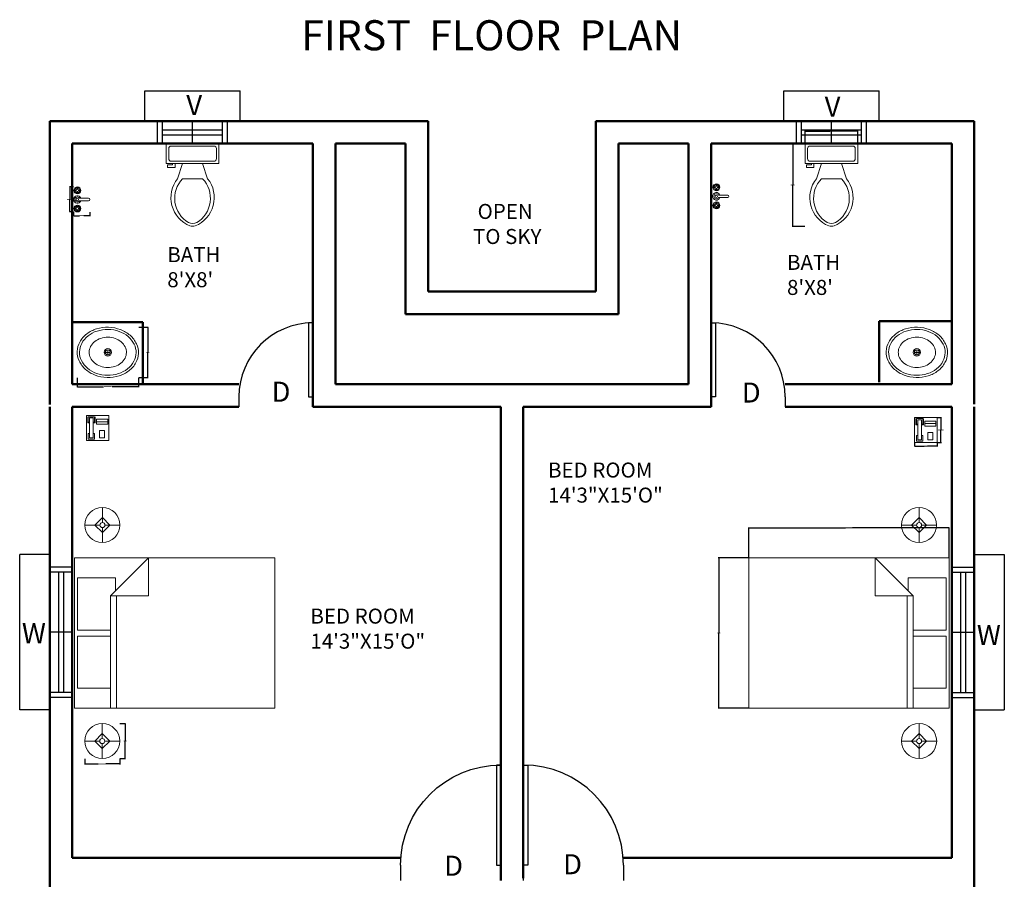
# Model space of a CAD drawing. Units: inches. Extents: x -8 to 1354, y -679 to 94.
# Tile 6 of 6: x 961 to 1354, y -249 to 94. Entities that reach past the tile are written whole.
import ezdxf

# ---------------------------------------------------------------- set-up
doc = ezdxf.new("R2010")
doc.units = ezdxf.units.IN
doc.header["$MEASUREMENT"] = 0
for name, color, linetype, lineweight in [('A-ANNO-DIMS', 2, 'Continuous', 18), ('A-ANNO-TEXT', 7, 'Continuous', 25), ('A-AREA-IDEN', 7, 'Continuous', 25), ('A-DOOR', 3, 'Continuous', 25), ('A-FLOR-FIXT', 8, 'Continuous', 18), ('A-FURN', 8, 'Continuous', 18), ('A-GLAZ', 4, 'Continuous', 25), ('A-WALL', 1, 'Continuous', 50)]:
    doc.layers.add(name, color=color, linetype=linetype, lineweight=lineweight)
doc.styles.get("Standard").update_dxf_attribs({"font": 'arial.ttf'})
doc.dimstyles.get("Standard").update_dxf_attribs({"dimtxt": 0.18, "dimasz": 0.18, "dimexe": 0.18, "dimexo": 0.0625, "dimgap": 0.09, "dimtad": 0, "dimtih": 1, "dimtoh": 1, "dimdec": 1, "dimzin": 0, "dimdsep": 46, "dimlunit": 4, "dimtxsty": 'Standard', "dimcen": 0.09, "dimclrd": 2, "dimclre": 3, "dimclrt": 6, "dimadec": 0, "dimazin": 0, "dimtfac": 1, "dimtdec": 1, "dimtofl": 0, "dimtmove": 0, "dimatfit": 3, "dimfxl": 1, "dimtfill": 2, "dimtfillclr": 4, "dimtolj": 1, "dimtzin": 0, "dimarcsym": 0})

# ---------------------------------------------------------------- blocks, each defined once
blk = doc.blocks.new('*U30')
for p, q in [((0, 0), (0, -6)), ((40, 0), (40, -6))]:
    blk.add_line(p, q)
blk.add_lwpolyline([(0, 0), (0, 40), (1.75, 40), (1.75, 0)], close=True)
blk.add_arc((0, 0), 40, 0, 90)
blk = doc.blocks.new('*U7')
for p, q in [((-750, 0), (-750, -100)), ((0, 0), (0, -100))]:
    blk.add_line(p, q)
blk.add_lwpolyline([(0, 0), (0, 750), (-43.75, 750), (-43.75, 0)], close=True)
blk.add_arc((0, 0), 750, 90, 180)
blk = doc.blocks.new('*U4')
for p, q in [((0, 0), (0, -100)), ((750, 0), (750, -100))]:
    blk.add_line(p, q)
blk.add_lwpolyline([(0, 0), (0, 750), (43.75, 750), (43.75, 0)], close=True)
blk.add_arc((0, 0), 750, 0, 90)
blk = doc.blocks.new('Toilet - top')
for p, q in [((9.5, -6), (9.5, -2)), ((-10, -8.5), (-8, -8.5)), ((-10, -9.5), (-10, -8.5)), ((-7, -9.5), (-10, -9.5)), ((-8, -8.5), (-8, -8)), ((-7, -8), (-7, -9.5)), ((-4, -8), (-6, -14)), ((4, -8), (6, -14)), ((4, -14), (-4, -14))]:
    blk.add_line(p, q)
blk.add_lwpolyline([(10.5, -8), (10.5, 0), (-10.5, 0), (-10.5, -8)], close=True)
for points in [[(-9.5, -2), (-9.5, -6)], [(8.5, -1), (-8.5, -1)], [(-8.5, -7), (8.5, -7)]]:
    blk.add_lwpolyline(points)
for centre, radius, start, end in [((-8.62, -1.88), 0.884, 81.8699, 188.1301), ((8.62, -1.88), 0.884, 351.8699, 98.1301), ((-8.62, -6.12), 0.884, 171.8699, 278.1301), ((8.62, -6.12), 0.884, 261.8699, 8.1301), ((3.52, -21.58), 12.17, 141.4691, 247.9714), ((4.2, -21.82), 11.33, 136.3677, 238.9468), ((-3.52, -21.58), 12.17, 292.0284, 38.5307), ((-4.2, -21.82), 11.33, 301.053, 43.6321), ((0, -27.88), 4, 245.7318, 294.2682), ((0, -29), 4, 254.8605, 285.1395)]:
    blk.add_arc(centre, radius, start, end)
blk = doc.blocks.new('Faucet - Bathroom top')
for p, q in [((-4.107, 0.125), (-4.375, 0.125)), ((-3.75, 0.4788), (-3.75, 0.75)), ((-3.5, 0.482), (-3.5, 0.75)), ((-3.1461, 0.125), (-2.875, 0.125)), ((3.143, 0.125), (2.875, 0.125)), ((3.5, 0.4788), (3.5, 0.75)), ((3.75, 0.482), (3.75, 0.75)), ((4.1039, 0.125), (4.375, 0.125)), ((-4.1039, -0.125), (-4.375, -0.125)), ((-3.75, -0.4821), (-3.75, -0.75)), ((-3.5, -0.4789), (-3.5, -0.75)), ((-3.143, -0.125), (-2.875, -0.125)), ((-0.5, -0.8639), (-0.5, -4.5)), ((0.5, -4.5), (0.5, -0.8631)), ((3.1461, -0.125), (2.875, -0.125)), ((3.5, -0.4821), (3.5, -0.75)), ((3.75, -0.4789), (3.75, -0.75)), ((4.107, -0.125), (4.375, -0.125))]:
    blk.add_line(p, q)
for centre, radius in [((-3.625, 0), 1.375), ((-4.625, 0), 0.2795), ((-3.625, 0), 0.5), ((-3.625, 1), 0.2795), ((-2.625, 0), 0.2795), ((0, 0), 0.5), ((3.625, 0), 1.375), ((2.625, 0), 0.2795), ((3.625, 0), 0.5), ((3.625, 1), 0.2795), ((4.625, 0), 0.2795), ((-3.625, -1), 0.2795), ((3.625, -1), 0.2795)]:
    blk.add_circle(centre, radius)
for centre, radius, start, end in [((-3.625, 0), 1, 105.2407, 164.2093), ((-3.625, 0), 1, 16.44125, 74.07887), ((0, 0), 1.5, 289.6514, 250.3603), ((0, 0), 1, 300.3431, 239.7554), ((3.625, 0), 1, 106.12, 164.0884), ((3.625, 0), 1, 16.23422, 73.90469), ((-3.625, 0), 1, 196.2342, 253.9047), ((-3.625, 0), 1, 286.12, 344.0884), ((3.625, 0), 1, 196.4413, 254.0789), ((3.625, 0), 1, 285.2407, 344.2093), ((0, -4.5), 0.5, 180, 0)]:
    blk.add_arc(centre, radius, start, end)
blk = doc.blocks.new('Sink - Oval top')
for p, q in [((-1, 0), (1, 0)), ((0, 1), (0, -1))]:
    blk.add_line(p, q)
for points in [[(-12.23, 0.39, 0.117634), (-11.46, -3.36, 0.104469), (-8.88, -6.8, 0.090016), (-5.08, -9.07, 0.08192), (-0.32, -10.02, 0.08192), (4.49, -9.38, 0.090016), (8.42, -7.36, 0.104469), (11.22, -4.09, 0.117634), (12.23, -0.39, 0.117634), (11.46, 3.36, 0.104469), (8.88, 6.8, 0.090016), (5.08, 9.07, 0.08192), (0.32, 10.02, 0.08192), (-4.49, 9.38, 0.090016), (-8.42, 7.36, 0.104469), (-11.22, 4.09, 0.117634)], [(-11.29, 0.16, 0.118622), (-10.52, -3.25, 0.104678), (-8.07, -6.36, 0.089562), (-4.54, -8.37, 0.081185), (-0.13, -9.15, 0.081185), (4.3, -8.49, 0.089562), (7.89, -6.58, 0.104678), (10.42, -3.55, 0.118622), (11.29, -0.16, 0.118622), (10.52, 3.25, 0.104678), (8.07, 6.36, 0.089562), (4.54, 8.37, 0.081185), (0.13, 9.15, 0.081185), (-4.3, 8.49, 0.089562), (-7.89, 6.58, 0.104678), (-10.42, 3.55, 0.118622)], [(-7.42, 0.08, 0.118283), (-6.91, -2.17, 0.104607), (-5.29, -4.21, 0.089718), (-2.97, -5.53, 0.081436), (-0.07, -6.04, 0.081436), (2.84, -5.59, 0.089718), (5.2, -4.33, 0.104607), (6.86, -2.32, 0.118283), (7.42, -0.08, 0.118283), (6.91, 2.17, 0.104607), (5.29, 4.21, 0.089718), (2.97, 5.53, 0.081436), (0.07, 6.04, 0.081436), (-2.84, 5.59, 0.089718), (-5.2, 4.33, 0.104607), (-6.86, 2.32, 0.118283)]]:
    blk.add_lwpolyline(points, format="xyb", close=True)
for radius in [1.5, 1]:
    blk.add_circle((0, 0), radius)
blk = doc.blocks.new('Bed - Queen')
for p, q in [((0, -80.00003), (0, 0)), ((0, 0), (59.99999, 0)), ((59.99999, 0), (59.99999, -80.00003)), ((7.99999, -1.2), (28.79998, -1.2)), ((7.99999, -14.4), (7.99999, -1.2)), ((28.79998, -1.2), (28.79998, -14.4)), ((31.19999, -1.2), (51.99999, -1.2)), ((31.19999, -14.4), (31.19999, -1.2)), ((51.99999, -1.2), (51.99999, -16.4)), ((0, -14.4), (44.8, -14.4)), ((59.99999, -29.6), (44.8, -14.4)), ((44.8, -14.4), (44.8, -29.6)), ((44.8, -16.8), (0, -16.8)), ((51.99999, -16.4), (46.79936, -16.4)), ((44.8, -29.6), (59.99999, -29.6)), ((59.99999, -80.00003), (0, -80.00003))]:
    blk.add_line(p, q)
blk = doc.blocks.new('Lamp - Table')
for p, q in [((0, 7), (0, 1)), ((-1, 0), (-7, 0)), ((0, 3), (-3, 0)), ((-3, 0), (0, -3)), ((3, 0), (0, 3)), ((0, -3), (3, 0)), ((1, 0), (7, 0)), ((0, -1), (0, -7))]:
    blk.add_line(p, q)
for radius in [7, 1]:
    blk.add_circle((0, 0), radius)
blk = doc.blocks.new('Phone - Desk')
for p, q in [((-4.5, -5), (-4.5, 5)), ((-4.5, 5), (4.5, 5)), ((-4, 4.5), (-4, 2)), ((-3.75, 4.5), (-3.75, 2.25)), ((-1.25, 4.5), (-3.75, 4.5)), ((-3.25, 4), (-3.25, -4)), ((-3.25, 4), (-1.75, 4)), ((-1.75, -4), (-1.75, 4)), ((-1.25, 2.25), (-1.25, 4.5)), ((-1, 2), (-1, 4.5)), ((4.5, 5), (4.5, -5)), ((-4, 2), (-3.25, 2)), ((-3.75, 2.25), (-3.25, 2.25)), ((-1.75, 2.25), (-1.25, 2.25)), ((-1.75, 2), (-1, 2)), ((4, 3.5), (-0.5, 3.5)), ((-0.5, 3.5), (-0.5, 1.5)), ((-0.5, 2.5), (4, 2.5)), ((-0.5, 1.5), (4, 1.5)), ((4, 1.5), (4, 3.5)), ((-3.75, -2.25), (-3.25, -2.25)), ((-3.75, -4.5), (-3.75, -2.25)), ((-1.75, -2.25), (-1.25, -2.25)), ((-1.25, -2.25), (-1.25, -4.5)), ((2.75, -1), (0.75, -1)), ((0.75, -1), (0.75, -4)), ((2.75, -4), (2.75, -1)), ((4.5, -5), (-4.5, -5)), ((-1.25, -4.5), (-3.75, -4.5)), ((-3.25, -4), (-1.75, -4)), ((0.75, -4), (2.75, -4))]:
    blk.add_line(p, q)
blk = doc.blocks.new('WIN-W')
at = {"ltscale": 2}
for p, q in [((12, 62), (0, 62)), ((0, 0), (0, 62)), ((12, 57), (12, 62)), ((12, 5), (12, 0)), ((12, 0), (0, 0))]:
    blk.add_line(p, q, dxfattribs=at)
for p, q in [((21, 57), (12, 57)), ((21, 5), (12, 5))]:
    blk.add_line(p, q)
blk = doc.blocks.new('VENT-V')
for p, q in [((0, 9), (0, 21)), ((0, 21), (38, 21)), ((38, 9), (38, 21)), ((5, 9), (0, 9)), ((5, 0), (5, 9)), ((33, 0), (33, 9)), ((33, 9), (38, 9))]:
    blk.add_line(p, q)
blk = doc.blocks.new('*D79')
at = {"layer": 'A-ANNO-DIMS', "color": 3, "lineweight": -2, "transparency": 16777216}
for p, q in [((986.72, -201.15), (986.72, -203.36)), ((1000.72, -201.15), (1000.72, -203.36))]:
    blk.add_line(p, q, dxfattribs=at)
at = {"layer": 'A-ANNO-DIMS', "color": 2, "lineweight": -2, "transparency": 16777216}
for p, q in [((986.9, -203.18), (992.27, -203.18)), ((1000.54, -203.18), (995.17, -203.18))]:
    blk.add_line(p, q, dxfattribs=at)
at = {"layer": 'A-ANNO-DIMS', "color": 2, "transparency": 16777216}
for points in [[(986.9, -203.15), (986.9, -203.21), (986.72, -203.18)], [(1000.54, -203.15), (1000.54, -203.21), (1000.72, -203.18)]]:
    blk.add_solid(points, dxfattribs=at)
at = {"layer": 'Defpoints', "color": 0, "transparency": 16777216}
for p in [(986.72, -201.08), (1000.72, -201.08), (1000.72, -203.18)]:
    blk.add_point(p, dxfattribs=at)
at = {"layer": 'A-ANNO-DIMS', "color": 6, "transparency": 16777216, "insert": (993.72, -203.18), "char_height": 0.18, "attachment_point": 5, "bg_fill": 1, "box_fill_scale": 1.25, "bg_fill_color": 4, "bg_fill_transparency": 0}
blk.add_mtext('\\A1;TABLE LAMP 1\'-2" TYP.', dxfattribs=at)
blk = doc.blocks.new('*D80')
at = {"layer": 'A-ANNO-DIMS', "color": 3, "lineweight": -2, "transparency": 16777216}
for p, q in [((1000.78, -187.08), (1003, -187.08)), ((1000.78, -201.08), (1003, -201.08))]:
    blk.add_line(p, q, dxfattribs=at)
at = {"layer": 'A-ANNO-DIMS', "color": 2, "lineweight": -2, "transparency": 16777216}
for p, q in [((1002.82, -187.26), (1002.82, -193.9)), ((1002.82, -200.9), (1002.82, -194.26))]:
    blk.add_line(p, q, dxfattribs=at)
at = {"layer": 'A-ANNO-DIMS', "color": 2, "transparency": 16777216}
for points in [[(1002.79, -187.26), (1002.85, -187.26), (1002.82, -187.08)], [(1002.79, -200.9), (1002.85, -200.9), (1002.82, -201.08)]]:
    blk.add_solid(points, dxfattribs=at)
at = {"layer": 'Defpoints', "color": 0, "transparency": 16777216}
for p in [(1000.72, -187.08), (1002.82, -187.08), (1000.72, -201.08)]:
    blk.add_point(p, dxfattribs=at)
at = {"layer": 'A-ANNO-DIMS', "color": 6, "transparency": 16777216, "insert": (1002.82, -194.08), "char_height": 0.18, "attachment_point": 5, "bg_fill": 1, "box_fill_scale": 1.25, "bg_fill_color": 4, "bg_fill_transparency": 0}
blk.add_mtext('\\A1;1\'-2" TYP.', dxfattribs=at)
blk = doc.blocks.new('*D85')
at = {"layer": 'A-ANNO-DIMS', "color": 3, "lineweight": -2, "transparency": 16777216}
for p, q in [((1251.81, -120.92), (1251.81, -108.8)), ((1331.81, -120.92), (1331.81, -108.8))]:
    blk.add_line(p, q, dxfattribs=at)
at = {"layer": 'A-ANNO-DIMS', "color": 2, "lineweight": -2, "transparency": 16777216}
for p, q in [((1251.99, -108.98), (1290.4, -108.98)), ((1331.63, -108.98), (1293.23, -108.98))]:
    blk.add_line(p, q, dxfattribs=at)
at = {"layer": 'A-ANNO-DIMS', "color": 2, "transparency": 16777216}
for points in [[(1251.99, -108.95), (1251.99, -109.01), (1251.81, -108.98)], [(1331.63, -108.95), (1331.63, -109.01), (1331.81, -108.98)]]:
    blk.add_solid(points, dxfattribs=at)
at = {"layer": 'Defpoints', "color": 0, "transparency": 16777216}
for p in [(1331.81, -108.98), (1251.81, -120.98), (1331.81, -120.98)]:
    blk.add_point(p, dxfattribs=at)
at = {"layer": 'A-ANNO-DIMS', "color": 6, "transparency": 16777216, "insert": (1291.81, -108.98), "char_height": 0.18, "attachment_point": 5, "bg_fill": 1, "box_fill_scale": 1.25, "bg_fill_color": 4, "bg_fill_transparency": 0}
blk.add_mtext('\\A1;QUEEN BED 6\'-8" TYP.', dxfattribs=at)
blk = doc.blocks.new('*D86')
at = {"layer": 'A-ANNO-DIMS', "color": 3, "lineweight": -2, "transparency": 16777216}
for p, q in [((1251.75, -120.98), (1239.63, -120.98)), ((1251.75, -180.98), (1239.63, -180.98))]:
    blk.add_line(p, q, dxfattribs=at)
at = {"layer": 'A-ANNO-DIMS', "color": 2, "lineweight": -2, "transparency": 16777216}
for p, q in [((1239.81, -121.16), (1239.81, -150.8)), ((1239.81, -180.8), (1239.81, -151.16))]:
    blk.add_line(p, q, dxfattribs=at)
at = {"layer": 'A-ANNO-DIMS', "color": 2, "transparency": 16777216}
for points in [[(1239.78, -121.16), (1239.84, -121.16), (1239.81, -120.98)], [(1239.78, -180.8), (1239.84, -180.8), (1239.81, -180.98)]]:
    blk.add_solid(points, dxfattribs=at)
at = {"layer": 'Defpoints', "color": 0, "transparency": 16777216}
for p in [(1239.81, -120.98), (1251.81, -120.98), (1251.81, -180.98)]:
    blk.add_point(p, dxfattribs=at)
at = {"layer": 'A-ANNO-DIMS', "color": 6, "transparency": 16777216, "insert": (1239.81, -150.98), "char_height": 0.18, "attachment_point": 5, "bg_fill": 1, "box_fill_scale": 1.25, "bg_fill_color": 4, "bg_fill_transparency": 0}
blk.add_mtext('\\A1;5\'-0" TYP.', dxfattribs=at)
blk = doc.blocks.new('*D89')
at = {"layer": 'A-ANNO-DIMS', "color": 3, "lineweight": -2, "transparency": 16777216}
for p, q in [((1327.05, -64.89), (1328.67, -64.89)), ((1327.05, -74.89), (1328.67, -74.89))]:
    blk.add_line(p, q, dxfattribs=at)
at = {"layer": 'A-ANNO-DIMS', "color": 2, "lineweight": -2, "transparency": 16777216}
for p, q in [((1328.49, -65.07), (1328.49, -69.7)), ((1328.49, -74.71), (1328.49, -70.07))]:
    blk.add_line(p, q, dxfattribs=at)
at = {"layer": 'A-ANNO-DIMS', "color": 2, "transparency": 16777216}
for points in [[(1328.46, -65.07), (1328.52, -65.07), (1328.49, -64.89)], [(1328.46, -74.71), (1328.52, -74.71), (1328.49, -74.89)]]:
    blk.add_solid(points, dxfattribs=at)
at = {"layer": 'Defpoints', "color": 0, "transparency": 16777216}
for p in [(1326.99, -64.89), (1328.49, -64.89), (1326.99, -74.89)]:
    blk.add_point(p, dxfattribs=at)
at = {"layer": 'A-ANNO-DIMS', "color": 6, "transparency": 16777216, "insert": (1328.49, -69.89), "char_height": 0.18, "attachment_point": 5, "bg_fill": 1, "box_fill_scale": 1.25, "bg_fill_color": 4, "bg_fill_transparency": 0}
blk.add_mtext('\\A1;PHONE 0\'-10" TYP.', dxfattribs=at)
blk = doc.blocks.new('*D90')
at = {"layer": 'A-ANNO-DIMS', "color": 3, "lineweight": -2, "transparency": 16777216}
for p, q in [((1317.99, -74.95), (1317.99, -76.57)), ((1326.99, -74.95), (1326.99, -76.57))]:
    blk.add_line(p, q, dxfattribs=at)
at = {"layer": 'A-ANNO-DIMS', "color": 2, "lineweight": -2, "transparency": 16777216}
for p, q in [((1318.17, -76.39), (1321.85, -76.39)), ((1326.81, -76.39), (1323.13, -76.39))]:
    blk.add_line(p, q, dxfattribs=at)
at = {"layer": 'A-ANNO-DIMS', "color": 2, "transparency": 16777216}
for points in [[(1318.17, -76.36), (1318.17, -76.42), (1317.99, -76.39)], [(1326.81, -76.36), (1326.81, -76.42), (1326.99, -76.39)]]:
    blk.add_solid(points, dxfattribs=at)
at = {"layer": 'Defpoints', "color": 0, "transparency": 16777216}
for p in [(1317.99, -74.89), (1326.99, -74.89), (1326.99, -76.39)]:
    blk.add_point(p, dxfattribs=at)
at = {"layer": 'A-ANNO-DIMS', "color": 6, "transparency": 16777216, "insert": (1322.49, -76.39), "char_height": 0.18, "attachment_point": 5, "bg_fill": 1, "box_fill_scale": 1.25, "bg_fill_color": 4, "bg_fill_transparency": 0}
blk.add_mtext('\\A1;0\'-9" TYP.', dxfattribs=at)
blk = doc.blocks.new('*D93')
at = {"layer": 'A-ANNO-DIMS', "color": 3, "lineweight": -2, "transparency": 16777216}
for p, q in [((983.67, -49.09), (983.67, -52.89)), ((1008.22, -49.09), (1008.22, -52.89))]:
    blk.add_line(p, q, dxfattribs=at)
at = {"layer": 'A-ANNO-DIMS', "color": 2, "lineweight": -2, "transparency": 16777216}
for p, q in [((983.85, -52.71), (994.27, -52.71)), ((1008.04, -52.71), (997.62, -52.71))]:
    blk.add_line(p, q, dxfattribs=at)
at = {"layer": 'A-ANNO-DIMS', "color": 2, "transparency": 16777216}
for points in [[(983.85, -52.68), (983.85, -52.74), (983.67, -52.71)], [(1008.04, -52.68), (1008.04, -52.74), (1008.22, -52.71)]]:
    blk.add_solid(points, dxfattribs=at)
at = {"layer": 'Defpoints', "color": 0, "transparency": 16777216}
for p in [(983.67, -49.02), (1008.22, -49.02), (1008.22, -52.71)]:
    blk.add_point(p, dxfattribs=at)
at = {"layer": 'A-ANNO-DIMS', "color": 6, "transparency": 16777216, "insert": (995.95, -52.71), "char_height": 0.18, "attachment_point": 5, "bg_fill": 1, "box_fill_scale": 1.25, "bg_fill_color": 4, "bg_fill_transparency": 0}
blk.add_mtext('\\A1;WASH BASIN 2\'-0 1/2" TYP.', dxfattribs=at)
blk = doc.blocks.new('*D94')
at = {"layer": 'A-ANNO-DIMS', "color": 3, "lineweight": -2, "transparency": 16777216}
for p, q in [((1008.29, -28.89), (1012.09, -28.89)), ((1008.29, -49.02), (1012.09, -49.02))]:
    blk.add_line(p, q, dxfattribs=at)
at = {"layer": 'A-ANNO-DIMS', "color": 2, "lineweight": -2, "transparency": 16777216}
for p, q in [((1011.91, -29.07), (1011.91, -38.77)), ((1011.91, -48.84), (1011.91, -39.14))]:
    blk.add_line(p, q, dxfattribs=at)
at = {"layer": 'A-ANNO-DIMS', "color": 2, "transparency": 16777216}
for points in [[(1011.88, -29.07), (1011.94, -29.07), (1011.91, -28.89)], [(1011.88, -48.84), (1011.94, -48.84), (1011.91, -49.02)]]:
    blk.add_solid(points, dxfattribs=at)
at = {"layer": 'Defpoints', "color": 0, "transparency": 16777216}
for p in [(1008.22, -28.89), (1011.91, -28.89), (1008.22, -49.02)]:
    blk.add_point(p, dxfattribs=at)
at = {"layer": 'A-ANNO-DIMS', "color": 6, "transparency": 16777216, "insert": (1011.91, -38.96), "char_height": 0.18, "attachment_point": 5, "bg_fill": 1, "box_fill_scale": 1.25, "bg_fill_color": 4, "bg_fill_transparency": 0}
blk.add_mtext('\\A1;1\'-8" TYP.', dxfattribs=at)
blk = doc.blocks.new('*D95')
at = {"layer": 'A-ANNO-DIMS', "color": 3, "lineweight": -2, "transparency": 16777216}
for p, q in [((1274.21, 44.35), (1269.14, 44.35)), ((1274.21, 11.31), (1269.14, 11.31))]:
    blk.add_line(p, q, dxfattribs=at)
at = {"layer": 'A-ANNO-DIMS', "color": 2, "lineweight": -2, "transparency": 16777216}
for p, q in [((1269.32, 44.17), (1269.32, 28.01)), ((1269.32, 11.49), (1269.32, 27.65))]:
    blk.add_line(p, q, dxfattribs=at)
at = {"layer": 'A-ANNO-DIMS', "color": 2, "transparency": 16777216}
for points in [[(1269.29, 44.17), (1269.35, 44.17), (1269.32, 44.35)], [(1269.29, 11.49), (1269.35, 11.49), (1269.32, 11.31)]]:
    blk.add_solid(points, dxfattribs=at)
at = {"layer": 'Defpoints', "color": 0, "transparency": 16777216}
for p in [(1269.32, 44.35), (1274.28, 44.35), (1274.28, 11.31)]:
    blk.add_point(p, dxfattribs=at)
at = {"layer": 'A-ANNO-DIMS', "color": 6, "transparency": 16777216, "insert": (1269.32, 27.83), "char_height": 0.18, "attachment_point": 5, "bg_fill": 1, "box_fill_scale": 1.25, "bg_fill_color": 4, "bg_fill_transparency": 0}
blk.add_mtext('\\A1;WC 2\'-9" TYP.', dxfattribs=at)
blk = doc.blocks.new('*D96')
at = {"layer": 'A-ANNO-DIMS', "color": 3, "lineweight": -2, "transparency": 16777216}
for p, q in [((1274.28, 44.42), (1274.28, 49.49)), ((1295.28, 44.42), (1295.28, 49.49))]:
    blk.add_line(p, q, dxfattribs=at)
at = {"layer": 'A-ANNO-DIMS', "color": 2, "lineweight": -2, "transparency": 16777216}
for p, q in [((1274.46, 49.31), (1284.15, 49.31)), ((1295.1, 49.31), (1285.41, 49.31))]:
    blk.add_line(p, q, dxfattribs=at)
at = {"layer": 'A-ANNO-DIMS', "color": 2, "transparency": 16777216}
for points in [[(1274.46, 49.34), (1274.46, 49.28), (1274.28, 49.31)], [(1295.1, 49.34), (1295.1, 49.28), (1295.28, 49.31)]]:
    blk.add_solid(points, dxfattribs=at)
at = {"layer": 'Defpoints', "color": 0, "transparency": 16777216}
for p in [(1295.28, 49.31), (1274.28, 44.35), (1295.28, 44.35)]:
    blk.add_point(p, dxfattribs=at)
at = {"layer": 'A-ANNO-DIMS', "color": 6, "transparency": 16777216, "insert": (1284.78, 49.31), "char_height": 0.18, "attachment_point": 5, "bg_fill": 1, "box_fill_scale": 1.25, "bg_fill_color": 4, "bg_fill_transparency": 0}
blk.add_mtext('\\A1;1\'-9" TYP.', dxfattribs=at)
blk = doc.blocks.new('*D97')
at = {"layer": 'A-ANNO-DIMS', "color": 3, "lineweight": -2, "transparency": 16777216}
for p, q in [((982.22, 27.06), (980.61, 27.06)), ((982.22, 17.06), (980.61, 17.06))]:
    blk.add_line(p, q, dxfattribs=at)
at = {"layer": 'A-ANNO-DIMS', "color": 2, "lineweight": -2, "transparency": 16777216}
for p, q in [((980.79, 26.88), (980.79, 22.25)), ((980.79, 17.24), (980.79, 21.88))]:
    blk.add_line(p, q, dxfattribs=at)
at = {"layer": 'A-ANNO-DIMS', "color": 2, "transparency": 16777216}
for points in [[(980.76, 26.88), (980.82, 26.88), (980.79, 27.06)], [(980.76, 17.24), (980.82, 17.24), (980.79, 17.06)]]:
    blk.add_solid(points, dxfattribs=at)
at = {"layer": 'Defpoints', "color": 0, "transparency": 16777216}
for p in [(980.79, 27.06), (982.29, 27.06), (982.29, 17.06)]:
    blk.add_point(p, dxfattribs=at)
at = {"layer": 'A-ANNO-DIMS', "color": 6, "transparency": 16777216, "insert": (980.79, 22.06), "char_height": 0.18, "attachment_point": 5, "bg_fill": 1, "box_fill_scale": 1.25, "bg_fill_color": 4, "bg_fill_transparency": 0}
blk.add_mtext('\\A1;FAUCET 0\'-10" TYP.', dxfattribs=at)
blk = doc.blocks.new('*D98')
at = {"layer": 'A-ANNO-DIMS', "color": 3, "lineweight": -2, "transparency": 16777216}
for p, q in [((982.29, 17), (982.29, 15.38)), ((988.79, 17), (988.79, 15.38))]:
    blk.add_line(p, q, dxfattribs=at)
at = {"layer": 'A-ANNO-DIMS', "color": 2, "lineweight": -2, "transparency": 16777216}
for p, q in [((982.47, 15.56), (984.69, 15.56)), ((988.61, 15.56), (986.39, 15.56))]:
    blk.add_line(p, q, dxfattribs=at)
at = {"layer": 'A-ANNO-DIMS', "color": 2, "transparency": 16777216}
for points in [[(982.47, 15.59), (982.47, 15.53), (982.29, 15.56)], [(988.61, 15.59), (988.61, 15.53), (988.79, 15.56)]]:
    blk.add_solid(points, dxfattribs=at)
at = {"layer": 'Defpoints', "color": 0, "transparency": 16777216}
for p in [(982.29, 17.06), (988.79, 17.06), (982.29, 15.56)]:
    blk.add_point(p, dxfattribs=at)
at = {"layer": 'A-ANNO-DIMS', "color": 6, "transparency": 16777216, "insert": (985.54, 15.56), "char_height": 0.18, "attachment_point": 5, "bg_fill": 1, "box_fill_scale": 1.25, "bg_fill_color": 4, "bg_fill_transparency": 0}
blk.add_mtext('\\A1;0\'-6 1/2" TYP.', dxfattribs=at)

msp = doc.modelspace()

# ---------------------------------------------------------------- linework, layer by layer
at = {"layer": 'A-GLAZ'}
for p, q in [((1017.78, 44.35), (1017.78, 53.35)), ((1029.78, 44.35), (1029.78, 53.35)), ((1041.78, 44.35), (1041.78, 53.35)), ((1272.78, 44.35), (1272.78, 53.35)), ((1284.78, 44.35), (1284.78, 53.35)), ((1296.78, 44.35), (1296.78, 53.35)), ((1017.78, 49.85), (1041.78, 49.85)), ((1017.78, 47.85), (1041.78, 47.85)), ((1272.78, 49.85), (1296.78, 49.85)), ((1272.78, 47.85), (1296.78, 47.85)), ((981.78, -126.65), (972.78, -126.65)), ((976.28, -126.65), (976.28, -174.65)), ((978.28, -126.65), (978.28, -174.65)), ((1332.78, -126.65), (1341.78, -126.65)), ((1336.28, -126.65), (1336.28, -174.65)), ((1338.28, -126.65), (1338.28, -174.65)), ((981.78, -150.65), (972.78, -150.65)), ((1332.78, -150.65), (1341.78, -150.65)), ((981.78, -174.65), (972.78, -174.65)), ((1332.78, -174.65), (1341.78, -174.65))]:
    msp.add_line(p, q, dxfattribs=at)
at = {"layer": 'A-WALL'}
for p, q in [((972.78, 53.35), (1086.78, 53.35)), ((972.78, -59.83), (972.78, 53.35)), ((1086.78, 53.35), (1123.78, 53.35)), ((1123.78, 53.35), (1123.78, -14.65)), ((1227.78, 53.35), (1190.78, 53.35)), ((1190.78, 53.35), (1190.78, -14.65)), ((1341.78, 53.35), (1227.78, 53.35)), ((1341.78, -59.69), (1341.78, 53.35)), ((981.78, 44.35), (1077.78, 44.35)), ((981.78, -51.65), (981.78, 44.35)), ((1077.78, 44.35), (1077.78, -60.65)), ((1086.78, 44.35), (1086.78, -51.65)), ((1086.78, 44.35), (1114.78, 44.35)), ((1114.78, 44.35), (1114.78, -23.65)), ((1227.78, 44.35), (1199.78, 44.35)), ((1199.78, 44.35), (1199.78, -23.65)), ((1227.78, 44.35), (1227.78, -51.65)), ((1332.78, 44.35), (1236.78, 44.35)), ((1236.78, 44.35), (1236.78, -60.65)), ((1332.78, -51.65), (1332.78, 44.35)), ((1190.78, -14.65), (1123.78, -14.65)), ((981.78, -26.86), (1009.86, -26.86)), ((1009.86, -26.86), (1009.86, -51.65)), ((1199.78, -23.65), (1114.78, -23.65)), ((1332.78, -26.5), (1303.85, -26.5)), ((1303.85, -26.5), (1303.85, -50.83)), ((1037.89, -51.65), (981.78, -51.65)), ((1048.25, -51.65), (981.78, -51.65)), ((1152.78, -51.65), (1086.78, -51.65)), ((1227.78, -51.65), (1152.78, -51.65)), ((1332.78, -51.65), (1266.3, -51.65)), ((972.78, -60.65), (972.78, -429.65)), ((1038.23, -60.65), (981.78, -60.65)), ((981.78, -60.65), (981.78, -240.65)), ((1048.25, -60.65), (981.78, -60.65)), ((1152.78, -60.65), (1077.78, -60.65)), ((1152.78, -249.65), (1152.78, -60.65)), ((1161.78, -248.83), (1161.78, -60.65)), ((1236.78, -60.65), (1161.78, -60.65)), ((1332.78, -60.65), (1266.3, -60.65)), ((1332.78, -240.65), (1332.78, -60.65)), ((1341.78, -248.83), (1341.78, -60.65)), ((981.78, -240.65), (1112.89, -240.65)), ((1201.66, -240.65), (1332.78, -240.65)), ((1341.78, -248.83), (1341.78, -333.65))]:
    msp.add_line(p, q, dxfattribs=at)

# ---------------------------------------------------------------- block references
at = {"layer": 'A-DOOR', "xscale": 0.0393700787401575, "yscale": 0.0393700787401575, "zscale": 0.0393700787401575}
for name, p in [('*U7', (1077.78, -56.71)), ('*U4', (1236.78, -56.71))]:
    msp.add_blockref(name, p, dxfattribs=at)
at = {"layer": 'A-DOOR', "xscale": -1}
msp.add_blockref('*U30', (1152.78, -243.65), dxfattribs=at)
at = {"layer": 'A-DOOR'}
msp.add_blockref('*U30', (1161.78, -243.65), dxfattribs=at)
at = {"layer": 'A-FLOR-FIXT'}
for name, p in [('Toilet - top', (1029.78, 44.35)), ('Toilet - top', (1284.78, 44.35)), ('Sink - Oval top', (995.95, -38.96)), ('Sink - Oval top', (1318.87, -38.96))]:
    msp.add_blockref(name, p, dxfattribs=at)
at = {"layer": 'A-FLOR-FIXT', "rotation": 90}
for p in [(1238.86, 23.3), (983.79, 22.06)]:
    msp.add_blockref('Faucet - Bathroom top', p, dxfattribs=at)
at = {"layer": 'A-FURN'}
for name, p in [('Phone - Desk', (991.91, -69.12)), ('Phone - Desk', (1322.49, -69.89)), ('Lamp - Table', (993.81, -107.87)), ('Lamp - Table', (993.72, -194.08))]:
    msp.add_blockref(name, p, dxfattribs=at)
at = {"layer": 'A-FURN', "xscale": -1}
for p in [(1319.77, -107.87), (1319.78, -194.08)]:
    msp.add_blockref('Lamp - Table', p, dxfattribs=at)
at = {"layer": 'A-FURN', "rotation": 90}
msp.add_blockref('Bed - Queen', (982.63, -180.98), dxfattribs=at)
at = {"layer": 'A-FURN', "xscale": -1, "rotation": 270}
msp.add_blockref('Bed - Queen', (1331.81, -180.98), dxfattribs=at)
at = {"layer": 'A-GLAZ'}
for name, p in [('VENT-V', (1010.78, 44.36)), ('VENT-V', (1265.78, 44.36)), ('WIN-W', (960.78, -181.64))]:
    msp.add_blockref(name, p, dxfattribs=at)
at = {"layer": 'A-GLAZ', "rotation": 180}
msp.add_blockref('WIN-W', (1353.78, -119.65), dxfattribs=at)

# ---------------------------------------------------------------- texts
at = {"layer": 'A-ANNO-TEXT', "attachment_point": 1}
for s, width, insert, char_height in [('FIRST  FLOOR  PLAN', 189.275, (1073.11, 93.58), 12), ('V', 71.0443, (1027.29, 63.7), 8), ('V', 71.0443, (1282.08, 63.08), 8), ('D', 71.0443, (1061.33, -50.67), 8), ('D', 71.0443, (1249.01, -50.99), 8), ('W', 71.0443, (961.65, -147.02), 8), ('W', 71.0443, (1342.81, -147.69), 8), ('D', 71.0443, (1177.7, -239.23), 8), ('D', 71.0443, (1130.21, -239.82), 8)]:
    msp.add_mtext_dynamic_manual_height_columns(s, width=width, gutter_width=1, heights=[0], dxfattribs=dict(at, insert=insert, char_height=char_height))
at = {"layer": 'A-AREA-IDEN', "char_height": 6, "attachment_point": 1}
for s, insert in [(' OPEN\\PTO SKY', (1141.71, 20.28)), ("BATH\\P8'X8'", (1019.69, 3.04)), ("BATH\\P8'X8'", (1267.05, -0.04)), ('BED ROOM\\P14\'3"X15\'O"', (1171.67, -82.92)), ('BED ROOM\\P14\'3"X15\'O"', (1076.81, -141.21))]:
    msp.add_mtext_dynamic_manual_height_columns(s, width=72.8194, gutter_width=1, heights=[0], dxfattribs=dict(at, insert=insert))

# ---------------------------------------------------------------- dimensions: what is measured, and where the dimension line sits
at = {"layer": 'A-ANNO-DIMS'}
for base, p1, p2, text, picture, middle in [((1295.28, 49.31), (1274.28, 44.35), (1295.28, 44.35), '<> TYP.', '*D96', (1284.78, 49.31)), ((1008.2239, -52.7075), (983.673, -49.0249), (1008.2239, -49.0249), 'WASH BASIN <> TYP.', '*D93', (995.9485, -52.7075)), ((1326.99, -76.39), (1317.99, -74.89), (1326.99, -74.89), '<> TYP.', '*D90', (1322.49, -76.39)), ((1331.81, -108.98), (1251.81, -120.98), (1331.81, -120.98), 'QUEEN BED <> TYP.', '*D85', (1291.81, -108.98)), ((1000.72, -203.18), (986.72, -201.08), (1000.72, -201.08), 'TABLE LAMP <> TYP.', '*D79', (993.72, -203.18))]:
    dim = msp.add_linear_dim(base=base, p1=p1, p2=p2, text=text, dimstyle='Standard', override={"dimdec": 1, "dimrnd": 0, "dimzin": 1, "dimlunit": 4, "dimfrac": 2}, dxfattribs=at)
    dim.commit()
    dim.dimension.update_dxf_attribs({"geometry": picture, "text_midpoint": middle})
for base, p1, p2, angle, text, picture, middle in [((1269.32, 44.35), (1274.28, 11.31), (1274.28, 44.35), 90, 'WC <> TYP.', '*D95', (1269.32, 27.83)), ((980.79, 27.06), (982.29, 17.06), (982.29, 27.06), 90, 'FAUCET <> TYP.', '*D97', (980.79, 22.06)), ((982.29, 15.56), (988.79, 17.06), (982.29, 17.06), 180, '<> TYP.', '*D98', (985.54, 15.56)), ((1011.91, -28.89), (1008.22, -49.02), (1008.22, -28.89), 90, '<> TYP.', '*D94', (1011.91, -38.96)), ((1328.49, -64.89), (1326.99, -74.89), (1326.99, -64.89), 90, 'PHONE <> TYP.', '*D89', (1328.49, -69.89)), ((1239.81, -120.98), (1251.81, -180.98), (1251.81, -120.98), 90, '<> TYP.', '*D86', (1239.81, -150.98)), ((1002.82, -187.08), (1000.72, -201.08), (1000.72, -187.08), 90, '<> TYP.', '*D80', (1002.82, -194.08))]:
    dim = msp.add_linear_dim(base=base, p1=p1, p2=p2, angle=angle, text=text, dimstyle='Standard', override={"dimdec": 1, "dimrnd": 0, "dimzin": 1, "dimlunit": 4, "dimfrac": 2}, dxfattribs=at)
    dim.commit()
    dim.dimension.update_dxf_attribs({"geometry": picture, "text_midpoint": middle})

doc.saveas('drawing.dxf')
